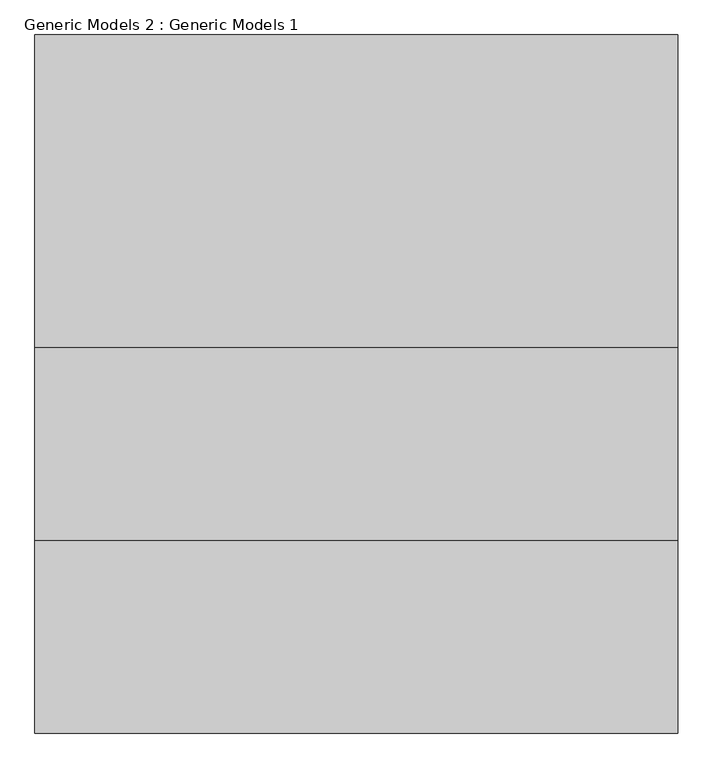
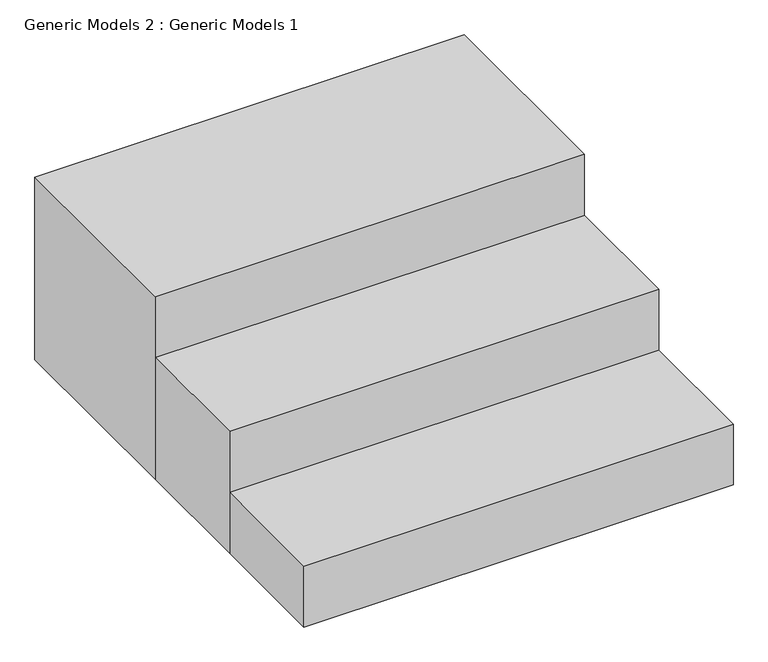
"""IFC4 building model written with IfcOpenShell, lengths in millimetres: proxy geometry, Generic Models 2 : Generic Models 1."""

from ifc_helpers import new_model, si_unit, frame, origin, place, context, project, spatial, polyline, outline, extrude, source, transform, mapped, element, save


def generic_models_2_generic_models_1_31704990(model_context):
    return source(origin(), model_context, "Body", "SweptSolid", [
        extrude(outline(polyline([(-7397.054995, 3753.3127283), (-7397.054995, 3260.3940862), (-8412.5002526, 3260.3940862), (-8412.5002526, 3753.3127283), (-7397.054995, 3753.3127283)])), frame((0.0, 0.0, -457.2), z_axis=(0.0, 0.0, 1.0), x_axis=(1.0, 0.0, 0.0)), (0.0, 0.0, 1.0), 457.2),
        extrude(outline(polyline([(-7397.054995, 3260.3940862), (-7397.054995, 2955.5940862), (-8412.5002526, 2955.5940862), (-8412.5002526, 3260.3940862), (-7397.054995, 3260.3940862)])), frame((0.0, 0.0, -457.2), z_axis=(0.0, 0.0, 1.0), x_axis=(1.0, 0.0, 0.0)), (0.0, 0.0, 1.0), 304.8),
        extrude(outline(polyline([(-7397.054995, 2955.5940862), (-7397.054995, 2650.7940862), (-8412.5002526, 2650.7940862), (-8412.5002526, 2955.5940862), (-7397.054995, 2955.5940862)])), frame((0.0, 0.0, -457.2), z_axis=(0.0, 0.0, 1.0), x_axis=(1.0, 0.0, 0.0)), (0.0, 0.0, 1.0), 152.4),
    ])


if __name__ == "__main__":
    model = new_model("IFC4")
    model_context = context("Model", 3, world=origin())
    ifc_project = project(units=[si_unit("LENGTHUNIT", "METRE", prefix="MILLI")], contexts=[model_context])
    site = spatial("IfcSite", under=ifc_project)
    building = spatial("IfcBuilding", under=site)
    placement = place(None, origin())
    generic_models_2_generic_models_1_shape = generic_models_2_generic_models_1_31704990(model_context)
    element("IfcBuildingElementProxy", 1, Name="Generic Models 2 : Generic Models 1", ObjectType="Generic Models 2 : Generic Models 1", at=placement, inside=building, context=model_context, shape_type="MappedRepresentation", body=[
        mapped(generic_models_2_generic_models_1_shape, transform((0.0, 0.0, 0.0), x_axis=(1.0, 0.0, 0.0), y_axis=(0.0, 1.0, 0.0), z_axis=(0.0, 0.0, 1.0))),
    ])
    save(model, "model.ifc")
